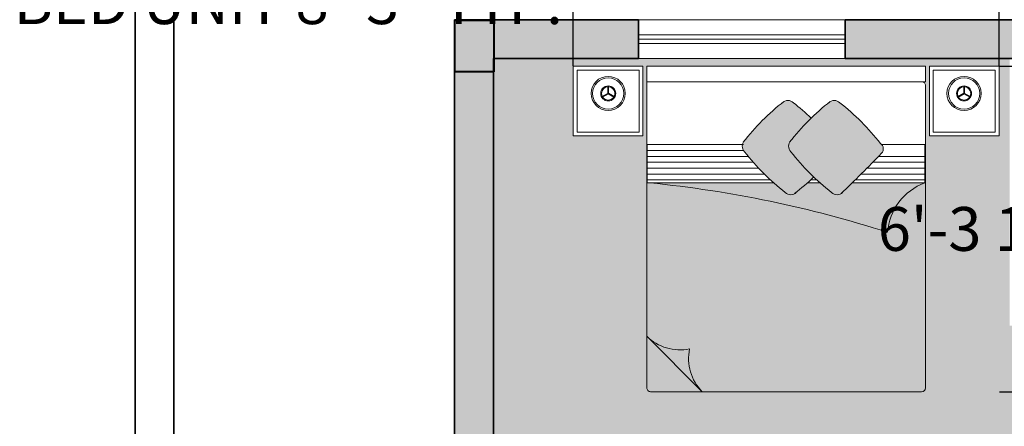
# Model space of a CAD drawing. Units: inches. Extents: x 1077 to 2505, y 1892 to 2728.
# Tile 12 of 26: x 1077 to 1306, y 2492 to 2586. Entities that reach past the tile are written whole.
import ezdxf

# ---------------------------------------------------------------- set-up
doc = ezdxf.new("R2010")
doc.units = ezdxf.units.IN
doc.linetypes.add('ACAD_ISO02W100', pattern=[15, 12, -3])
doc.layers.get('Defpoints').update_dxf_attribs({"color": 220, "linetype": 'ACAD_ISO02W100'})
for name, color, linetype, lineweight in [('00 FURNITURE', 15, 'Continuous', 15), ('A-ANNO-DIMS', 2, 'Continuous', 18), ('A-ANNO-TTLB', 7, 'Continuous', 35), ('A-COLS', 7, 'Continuous', 40), ('A-WALL-PATT', 7, 'Continuous', 9), ('WALL', 7, 'Continuous', 35), ('WINDOW', 160, 'Continuous', 13)]:
    doc.layers.add(name, color=color, linetype=linetype, lineweight=lineweight)
doc.layers.add('A-FLOR-PATT', color=254, linetype='Continuous', lineweight=9, true_color=0xd7ebd2)
doc.layers.add('A-FURN-PATT', color=177, linetype='Continuous', lineweight=9, true_color=0x293189)
doc.styles.get("Standard").update_dxf_attribs({"font": 'arial.ttf'})
doc.dimstyles.get("Standard").update_dxf_attribs({"dimtxt": 10.18, "dimasz": 0.18, "dimexe": 0.18, "dimexo": 0.0625, "dimgap": 0.09, "dimtad": 0, "dimtih": 1, "dimtoh": 1, "dimdec": 0, "dimzin": 0, "dimdsep": 46, "dimlunit": 3, "dimtxsty": 'Standard', "dimcen": 0.09, "dimadec": 0, "dimazin": 0, "dimtfac": 1, "dimtdec": 0, "dimtofl": 0, "dimtmove": 0, "dimatfit": 3, "dimfxl": 1, "dimtolj": 1, "dimtzin": 0, "dimarcsym": 0})

# ---------------------------------------------------------------- blocks, each defined once
blk = doc.blocks.new('RGWTG')
at = {"layer": '00 FURNITURE'}
for p, q in [((578.23, 3473.51), (577.36, 3475.01)), ((578.36, 3473.58), (577.49, 3475.09)), ((578.23, 3473.58), (577.36, 3472.08)), ((578.36, 3473.51), (577.49, 3472)), ((578.29, 3473.62), (580.03, 3473.62)), ((578.29, 3473.47), (580.03, 3473.47)), ((521.93, 3464.58), (509.03, 3451.68)), ((509.03, 3422.63), (509.03, 3463.68)), ((509.93, 3464.58), (566.4, 3464.58)), ((557.53, 3463.84), (557.53, 3464.49)), ((557.53, 3464.49), (566.4, 3464.49)), ((558.2, 3464.49), (558.2, 3435.82)), ((559.57, 3464.49), (559.57, 3437.25)), ((560.94, 3464.49), (560.94, 3438.58)), ((562.3, 3464.49), (562.3, 3439.83)), ((563.67, 3464.49), (563.67, 3440.99)), ((565.04, 3464.49), (565.04, 3442.08)), ((566.4, 3464.58), (580.98, 3464.58)), ((566.4, 3464.49), (566.4, 3442.08)), ((566.4, 3464.49), (566.4, 3463.84)), ((580.98, 3464.58), (580.98, 3416.72)), ((558.2, 3426.48), (558.2, 3425.04)), ((509.03, 3400.68), (509.03, 3422.63)), ((558.2, 3416.13), (558.2, 3399.95)), ((580.98, 3416.72), (580.98, 3400.68)), ((559.57, 3414.75), (559.57, 3399.95)), ((560.94, 3413.39), (560.94, 3399.95)), ((562.3, 3412.04), (562.3, 3399.95)), ((563.67, 3410.72), (563.67, 3399.95)), ((580.08, 3399.78), (509.93, 3399.78)), ((557.53, 3399.95), (557.53, 3400.6)), ((566.4, 3399.95), (557.53, 3399.95)), ((566.4, 3400.6), (566.4, 3399.95)), ((578.23, 3390.78), (577.36, 3392.29)), ((578.36, 3390.86), (577.49, 3392.36)), ((578.23, 3390.86), (577.36, 3389.36)), ((578.36, 3390.78), (577.49, 3389.28)), ((578.29, 3390.9), (580.03, 3390.9)), ((578.29, 3390.74), (580.03, 3390.74))]:
    blk.add_line(p, q, dxfattribs=at)
for points in [[(568.43, 3465.48), (584.63, 3465.48), (584.63, 3481.68), (568.43, 3481.68)], [(569.33, 3466.38), (583.73, 3466.38), (583.73, 3480.78), (569.33, 3480.78)], [(580.98, 3399.78), (584.63, 3399.78), (584.63, 3464.58), (580.98, 3464.58)], [(568.43, 3398.88), (584.63, 3398.88), (584.63, 3382.68), (568.43, 3382.68)], [(569.33, 3397.98), (583.73, 3397.98), (583.73, 3383.58), (569.33, 3383.58)]]:
    blk.add_lwpolyline(points, close=True, dxfattribs=at)
for points in [[(566.52, 3464.49), (557.53, 3464.49), (557.53, 3435.08)], [(557.53, 3427.21), (557.53, 3424.3)], [(557.53, 3416.82), (557.53, 3399.95), (566.4, 3399.95), (566.4, 3409.94)]]:
    blk.add_lwpolyline(points, dxfattribs=at)
for centre, radius in [((578.29, 3473.54), 3.97), ((578.29, 3473.54), 3.63), ((578.29, 3473.54), 1.74), ((578.29, 3473.54), 1.56), ((578.29, 3390.82), 3.97), ((578.29, 3390.82), 3.63), ((578.29, 3390.82), 1.74), ((578.29, 3390.82), 1.56)]:
    blk.add_circle(centre, radius, dxfattribs=at)
for centre, radius, start, end in [((509.93, 3463.68), 0.9, 90, 180), ((529.65, 3456.88), 10.9, 135.0361, 191.9278), ((290.56, 3490.52), 268.3, 342.2214, 354.2925), ((516.73, 3443.97), 10.9, 78.0722, 134.9639), ((566.05, 3440.57), 1.82, 45, 135), ((598.15, 3399.01), 54.32, 127.931, 142.069), ((533.58, 3399.31), 54.32, 37.931, 52.069), ((556.59, 3431.11), 1.82, 135, 225), ((598.15, 3388.23), 54.32, 127.931, 142.069), ((566.05, 3429.78), 1.82, 45, 135), ((533.58, 3388.53), 54.32, 37.931, 52.069), ((574.84, 3431.77), 1.82, 315, 45), ((597.87, 3463.6), 54.32, 217.931, 224.141), ((533.28, 3463.88), 54.32, 316.32, 322.069), ((574.84, 3420.99), 1.82, 315, 45), ((556.59, 3420.33), 1.82, 135, 225), ((533.28, 3453.1), 54.32, 307.931, 322.069), ((765.33, 3619.75), 290.45, 223.6069, 226.2326), ((545.02, 3395.29), 13.35, 20.4224, 85.5825), ((565.44, 3411.05), 1.47, 225.9674, 326.8337), ((509.93, 3400.68), 0.9, 180, 270), ((580.08, 3400.68), 0.9, 270, 0)]:
    blk.add_arc(centre, radius, start, end, dxfattribs=at)
blk = doc.blocks.new('C1')
h = blk.add_hatch(color=256)
h.dxf.hatch_style = 1
h.paths.add_polyline_path([(1668.56, 2445.41), (1677.56, 2445.41), (1677.56, 2457.41), (1668.56, 2457.41)])
for p, q in [((1668.56, 2457.41), (1677.56, 2457.41)), ((1668.56, 2445.41), (1668.56, 2457.41)), ((1677.56, 2457.41), (1677.56, 2445.41)), ((1677.56, 2445.41), (1668.56, 2445.41))]:
    blk.add_line(p, q)
blk = doc.blocks.new('WINDOW-48-EXT')
for p, q in [((0, 48), (0, 0)), ((3.5, 48), (3.5, 0)), ((4.5, 48), (4.5, 0)), ((5.5, 48), (5.5, 0)), ((9, 0), (9, 48))]:
    blk.add_line(p, q)
blk = doc.blocks.new('SHEET-FRAME-RESIDENTIAL')
for points in [[(0, 830.04), (543.52, 830.04), (543.52, 0), (0, 0)], [(9, 821.04), (534.52, 821.04), (534.52, 9), (9, 9)]]:
    blk.add_lwpolyline(points, close=True)
blk = doc.blocks.new('*D32')
at = {"layer": 'A-ANNO-DIMS', "color": 0, "lineweight": -2, "transparency": 16777216}
for p, q in [((1206.09, 2590.23), (1205.91, 2590.23)), ((1206.09, 2575.45), (1206.09, 2590.41)), ((1304.91, 2590.23), (1206.27, 2590.23)), ((1305.09, 2575.45), (1305.09, 2590.41))]:
    blk.add_line(p, q, dxfattribs=at)
at = {"layer": 'A-ANNO-DIMS', "color": 0, "transparency": 16777216}
for points in [[(1206.27, 2590.26), (1206.27, 2590.2), (1206.09, 2590.23)], [(1304.91, 2590.26), (1304.91, 2590.2), (1305.09, 2590.23)]]:
    blk.add_solid(points, dxfattribs=at)
at = {"layer": 'Defpoints', "color": 0, "transparency": 16777216}
for p in [(1206.09, 2590.23), (1206.09, 2575.38), (1305.09, 2575.38)]:
    blk.add_point(p, dxfattribs=at)
at = {"layer": 'A-ANNO-DIMS', "color": 0, "transparency": 16777216, "insert": (1139.85, 2590.23), "char_height": 10.18, "attachment_point": 5}
blk.add_mtext('\\A1;BED UNIT 8\'-3" TYP.', dxfattribs=at)
blk = doc.blocks.new('*D33')
at = {"layer": 'A-ANNO-DIMS', "color": 0, "lineweight": -2, "transparency": 16777216}
for p, q in [((1305.15, 2575.38), (1320.12, 2575.38)), ((1319.94, 2575.2), (1319.94, 2542.94)), ((1319.94, 2499.96), (1319.94, 2532.23)), ((1305.15, 2499.78), (1320.12, 2499.78))]:
    blk.add_line(p, q, dxfattribs=at)
at = {"layer": 'A-ANNO-DIMS', "color": 0, "transparency": 16777216}
for points in [[(1319.91, 2575.2), (1319.97, 2575.2), (1319.94, 2575.38)], [(1319.91, 2499.96), (1319.97, 2499.96), (1319.94, 2499.78)]]:
    blk.add_solid(points, dxfattribs=at)
at = {"layer": 'Defpoints', "color": 0, "transparency": 16777216}
for p in [(1305.09, 2575.38), (1319.94, 2575.38), (1305.09, 2499.78)]:
    blk.add_point(p, dxfattribs=at)
at = {"layer": 'A-ANNO-DIMS', "color": 0, "transparency": 16777216, "insert": (1319.94, 2537.58), "char_height": 10.18, "attachment_point": 5}
blk.add_mtext('\\A1;6\'-3 1/2" TYP.', dxfattribs=at)

msp = doc.modelspace()

# ---------------------------------------------------------------- hatches: boundary and pattern name
at = {"layer": 'A-FLOR-PATT', "transparency": 33554559}
h = msp.add_hatch(color=256, dxfattribs=at)
h.dxf.hatch_style = 1
h.paths.add_polyline_path([(1395.53, 2577.16), (1374.83, 2577.16), (1350.83, 2577.19), (1350.83, 2577.16), (1329.53, 2577.16), (1329.53, 2480.16), (1329.53, 2469.16), (1325.53, 2469.16), (1325.53, 2515.13), (1307.53, 2515.13), (1307.53, 2577.16), (1269.31, 2577.16), (1221.31, 2577.15), (1221.31, 2577.16), (1187.53, 2577.16), (1187.53, 2433.16), (1289.53, 2433.16), (1289.53, 2429.16), (1263.53, 2429.16), (1187.53, 2429.16), (1187.53, 2395.02), (1187.53, 2395.02), (1187.53, 2371.02), (1187.53, 2371.02), (1187.53, 2307.16), (1259.53, 2307.16), (1259.53, 2399.16), (1263.53, 2399.16), (1263.53, 2307.16), (1289.53, 2307.16), (1289.53, 2306.23), (1325.53, 2306.23), (1325.53, 2307.16), (1329.53, 2307.16), (1329.53, 2306.23), (1365.53, 2306.23), (1365.53, 2307.16), (1432.53, 2307.16), (1432.53, 2088.16), (1547.53, 2088.16), (1547.53, 2140.08), (1511.53, 2140.08), (1511.53, 2267.16), (1475.53, 2267.16), (1475.53, 2303.16), (1468.53, 2303.16), (1468.53, 2307.16), (1547.53, 2307.16), (1547.53, 2348.22), (1547.53, 2396.22), (1547.53, 2429.16), (1435.53, 2429.16), (1435.53, 2433.16), (1476.35, 2433.16), (1476.35, 2451.18), (1547.53, 2451.18), (1547.53, 2577.16), (1499.53, 2577.16), (1499.53, 2586.16), (1547.53, 2586.16), (1547.53, 2642.16), (1518.18, 2642.16), (1518.18, 2642.05), (1494.15, 2642.05), (1494.15, 2642.16), (1469.53, 2642.16), (1469.53, 2577.16), (1399.53, 2577.16), (1399.53, 2429.16), (1325.53, 2429.16), (1325.53, 2433.16), (1329.53, 2433.16), (1395.53, 2433.16), (1395.53, 2480.16), (1359.53, 2480.16), (1359.53, 2484.16), (1395.53, 2484.16)])
h.paths.add_polyline_path([(1357.65, 2482.07), (1355.65, 2482.07), (1355.65, 2481.07, 0.414214), (1356.65, 2480.07), (1344.65, 2480.07), (1344.65, 2477.06), (1343.27, 2477.06), (1343.27, 2480.07), (1330.65, 2480.07, -0.414214), (1329.65, 2481.07), (1329.65, 2484.07), (1331.65, 2484.07), (1331.65, 2510.07, -0.446908)], flags=16)
h.paths.add_polyline_path([(1305.09, 2559.18), (1288.89, 2559.18), (1288.89, 2575.38), (1305.09, 2575.38)], flags=16)
h.paths.add_polyline_path([(1304.19, 2560.08), (1289.79, 2560.08), (1289.79, 2574.48), (1304.19, 2574.48)], flags=0)
h.paths.add_polyline_path([(1287.99, 2500.68, -0.414214), (1287.09, 2499.78), (1265.14, 2499.78), (1224.09, 2499.78, -0.414214), (1223.19, 2500.68), (1223.19, 2557.16), (1223.19, 2571.74), (1223.19, 2575.38), (1287.99, 2575.38), (1287.99, 2571.74), (1287.09, 2571.74, -0.414214), (1287.99, 2570.84)], flags=16)
h.paths.add_polyline_path([(1292.98, 2569.05, -1), (1300.92, 2569.05, -1)], flags=0)
h.paths.add_polyline_path([(1293.32, 2569.05, -1), (1300.58, 2569.05, -1)], flags=0)
h.paths.add_polyline_path([(1322.8, 2462.21), (1322.8, 2431.71), (1323.05, 2430.71), (1323.05, 2431.71), (1321.8, 2431.71), (1321.8, 2462.19, 0.404641), (1292.3, 2431.71), (1292.05, 2430.71, -0.414214), (1291.55, 2430.21), (1291.05, 2430.21), (1291.05, 2429.71, -0.414214), (1290.55, 2429.21), (1289.55, 2429.21), (1289.55, 2434.21), (1290.55, 2434.21, -0.414214), (1291.05, 2433.71), (1291.05, 2433.21), (1291.55, 2433.21, -0.414214), (1292.05, 2432.71), (1292.3, 2431.71, -0.414214)], flags=16)
h.paths.add_polyline_path([(1287.82, 2548.28, 0.292232), (1279.17, 2536.8, 0.052719), (1223.93, 2548.28), (1223.28, 2548.28), (1223.28, 2557.16), (1223.93, 2557.16), (1245.42, 2557.16, -0.117785), (1245.77, 2557.93, -0.059418), (1254.87, 2567.02, -0.379859), (1257.28, 2566.88, -0.02509), (1261.41, 2563.32, -0.025935), (1265.65, 2567.02, -0.379859), (1268.06, 2566.88, -0.061767), (1277.52, 2557.43, -0.069393), (1277.82, 2557.16), (1287.82, 2557.16)], flags=0)
h.paths.add_polyline_path([(1263.47, 2548.28), (1260.56, 2548.28, -0.015371), (1258.01, 2546.13, -0.429576), (1255.37, 2546.06, -0.016036), (1252.69, 2548.28), (1223.28, 2548.28), (1223.28, 2554.42), (1246.78, 2554.42, 0.055344), (1255.37, 2546.06, 0.331768), (1257.52, 2545.74, 0.027343), (1262, 2549.64, 0.00919)], flags=0)
h.paths.add_polyline_path([(1295.56, 2568.34), (1296.87, 2569.09), (1296.87, 2570.6, 0.399698), (1295.39, 2569.05, 0.119004)], flags=0)
h.paths.add_polyline_path([(1295.21, 2569.05, -1), (1298.68, 2569.05, -1)], flags=0)
h.paths.add_polyline_path([(1296.95, 2568.96), (1297.03, 2569), (1297.03, 2569.09), (1296.99, 2569.11), (1296.91, 2568.98)], flags=0)
h.paths.add_polyline_path([(1402.28, 2462.19, -0.414214), (1432.78, 2431.69), (1433.03, 2432.69), (1432.78, 2431.69, 0.404641), (1403.28, 2462.17), (1403.28, 2431.69), (1402.03, 2431.69), (1402.03, 2430.69, -0.414214), (1401.53, 2430.19), (1401.03, 2430.19), (1401.03, 2429.69, -0.414214), (1400.53, 2429.19), (1399.53, 2429.19), (1399.53, 2434.19), (1400.53, 2434.19, -0.414214), (1401.03, 2433.69), (1401.03, 2433.19), (1401.53, 2433.19, -0.414214), (1402.03, 2432.69)], flags=16)
h.paths.add_polyline_path([(1470.16, 2535.21, -0.414214), (1471.06, 2536.11), (1527.54, 2536.11), (1542.12, 2536.11), (1545.76, 2536.11), (1545.76, 2471.31), (1542.12, 2471.31), (1542.12, 2472.21, -0.414214), (1541.22, 2471.31), (1471.06, 2471.31, -0.414214), (1470.16, 2472.21), (1470.16, 2494.16)], flags=16)
h.paths.add_polyline_path([(1483.07, 2536.11, 0.253465), (1480.11, 2526.15, 0.2538), (1470.15, 2523.19)], flags=16)
h.paths.add_polyline_path([(1223.19, 2512.69, 0.253465), (1233.14, 2509.74, 0.2538), (1236.1, 2499.77)], flags=16)
h.paths.add_polyline_path([(1469.77, 2578.72), (1469.77, 2581.72), (1471.77, 2581.72), (1471.77, 2607.72, -0.01951), (1473.77, 2607.68), (1473.77, 2579.72), (1473.77, 2578.72, -0.414214), (1472.77, 2577.72), (1470.77, 2577.72, -0.414214)], flags=16)
h.paths.add_polyline_path([(1382.46, 2398.13), (1395.04, 2398.13), (1395.04, 2399.74), (1382.46, 2399.74)], flags=16)
h.paths.add_polyline_path([(1379.94, 2397.18), (1379.94, 2389.82), (1380.5, 2389.82), (1380.5, 2396.05, -0.41429), (1381.06, 2396.61), (1396.47, 2396.61, -0.414213), (1397.03, 2396.05), (1397.03, 2389.82), (1397.59, 2389.82), (1397.59, 2397.18)], flags=16)
h.paths.add_polyline_path([(1263.37, 2428.14), (1263.37, 2426.14, -0.414214), (1262.37, 2425.14), (1261.37, 2425.14), (1233.41, 2425.14, 0.400854), (1259.37, 2401.04), (1259.37, 2401.14), (1261.37, 2401.14, -0.446908), (1233.37, 2427.14), (1259.37, 2427.14), (1259.37, 2429.14), (1262.37, 2429.14, -0.414214)], flags=16)
h.paths.add_polyline_path([(1404.79, 2398.13), (1417.37, 2398.13), (1417.37, 2399.74), (1404.79, 2399.74)], flags=16)
h.paths.add_polyline_path([(1402.27, 2397.18), (1404.79, 2398.13), (1417.37, 2398.13), (1419.92, 2397.18)], flags=16)
h.paths.add_polyline_path([(1432.26, 2383.16), (1432.26, 2370.59), (1433.87, 2370.59), (1433.87, 2383.16)], flags=16)
h.paths.add_polyline_path([(1431.3, 2385.69), (1423.84, 2385.69), (1423.84, 2385.13), (1430.18, 2385.13, -0.41429), (1430.74, 2384.57), (1430.74, 2369.16, -0.414237), (1430.18, 2368.6), (1423.84, 2368.6), (1423.84, 2368.03), (1431.3, 2368.03)], flags=16)
h.paths.add_polyline_path([(1417.37, 2351.16), (1417.37, 2349.54), (1418.9, 2349.54, 0.414236), (1419.92, 2350.56), (1419.92, 2352.11)], flags=16)
h.paths.add_polyline_path([(1395.04, 2351.16), (1395.04, 2349.54), (1396.58, 2349.54, 0.414235), (1397.59, 2350.56), (1397.59, 2352.11)], flags=16)
h.paths.add_polyline_path([(1366.7, 2370.05), (1365.09, 2370.05), (1365.09, 2368.52, 0.414235), (1366.11, 2367.5), (1367.66, 2367.5)], flags=16)
h.paths.add_polyline_path([(1419.36, 2359.47), (1419.36, 2353.24, -0.41419), (1418.8, 2352.68), (1403.39, 2352.68, -0.414137), (1402.83, 2353.24), (1402.83, 2359.47), (1397.03, 2359.47), (1397.03, 2353.24, -0.414189), (1396.47, 2352.68), (1381.06, 2352.68, -0.414137), (1380.5, 2353.24), (1380.5, 2359.47)], flags=16)
h.paths.add_polyline_path([(1222.29, 2559.18), (1206.09, 2559.18), (1206.09, 2575.38), (1222.29, 2575.38)], flags=16)
h.paths.add_polyline_path([(1221.39, 2560.08), (1206.99, 2560.08), (1206.99, 2574.48), (1221.39, 2574.48)], flags=0)
h.paths.add_polyline_path([(1482, 2577.72), (1482, 2580.73), (1483.38, 2580.73), (1483.38, 2577.72), (1484.77, 2577.72), (1484.77, 2574.72), (1483.38, 2574.72), (1483.38, 2577.72)], flags=16)
h.paths.add_polyline_path([(1266.37, 2415.53), (1266.37, 2414.14), (1263.37, 2414.14), (1263.37, 2415.53), (1260.36, 2415.53), (1260.36, 2416.91), (1263.37, 2416.91), (1263.37, 2415.53)], flags=16)
h.paths.add_polyline_path([(1210.26, 2569.05, -1), (1218.19, 2569.05, -1)], flags=0)
h.paths.add_polyline_path([(1210.6, 2569.05, -1), (1217.85, 2569.05, -1)], flags=0)
h.paths.add_polyline_path([(1212.84, 2568.34), (1214.15, 2569.09), (1214.15, 2570.6, 0.399698), (1212.67, 2569.05, 0.119004)], flags=0)
h.paths.add_polyline_path([(1212.49, 2569.05, -1), (1215.96, 2569.05, -1)], flags=0)
h.paths.add_polyline_path([(1214.23, 2568.96), (1214.3, 2568.91), (1214.3, 2569)], flags=0)
h.paths.add_polyline_path([(1507.18, 2480.12, 0.052719), (1518.66, 2535.36), (1518.66, 2536.01), (1527.54, 2536.01), (1527.54, 2535.36), (1527.54, 2513.88, -0.117785), (1528.31, 2513.53, -0.059418), (1537.4, 2504.43, -0.379859), (1537.26, 2502.01, -0.02509), (1533.7, 2497.89, -0.025935), (1537.4, 2493.64, -0.379859), (1537.26, 2491.23, -0.061767), (1527.8, 2481.77, -0.069393), (1527.54, 2481.47), (1527.54, 2471.47), (1518.66, 2471.47, 0.292232)], flags=0)
h.paths.add_polyline_path([(1516.43, 2503.92, -0.016036), (1518.66, 2506.6), (1518.66, 2536.01), (1524.8, 2536.01), (1524.8, 2512.51, 0.055344), (1516.43, 2503.92, 0.331768), (1516.12, 2501.77, 0.027343), (1520.01, 2497.29, 0.00919), (1518.66, 2495.82), (1518.66, 2498.73, -0.015371), (1516.5, 2501.28, -0.429576)], flags=0)
h.paths.add_polyline_path([(1499.63, 2625.5, -0.171636), (1502.82, 2631.01), (1502.82, 2633.37), (1498.68, 2633.37, -0.414214), (1497.7, 2634.36), (1497.7, 2640.66, -0.414214), (1498.68, 2641.64), (1514.82, 2641.64, -0.414214), (1515.81, 2640.66), (1515.81, 2634.36, -0.414214), (1514.82, 2633.37), (1510.69, 2633.37), (1510.69, 2631.01, -0.171636), (1513.88, 2625.5, -0.258205), (1509.31, 2614.47), (1504.19, 2614.47, -0.258205)], flags=16)
h.paths.add_polyline_path([(1501.2, 2625.5, -0.171636), (1504.39, 2631.01), (1509.12, 2631.01, -0.171636), (1512.3, 2625.5, -0.210384), (1509.35, 2616.02), (1504.16, 2616.02, -0.210384)], flags=0)
h.paths.add_polyline_path([(1529.56, 2537.01), (1529.56, 2553.21), (1545.76, 2553.21), (1545.76, 2537.01)], flags=16)
h.paths.add_polyline_path([(1530.46, 2537.91), (1530.46, 2552.31), (1544.86, 2552.31), (1544.86, 2537.91)], flags=0)
h.paths.add_polyline_path([(1535.45, 2545.07, -1), (1543.39, 2545.07, -1)], flags=0)
h.paths.add_polyline_path([(1535.8, 2545.07, -1), (1543.05, 2545.07, -1)], flags=0)
h.paths.add_polyline_path([(1529.56, 2470.41), (1545.76, 2470.41), (1545.76, 2454.21), (1529.56, 2454.21)], flags=16)
h.paths.add_polyline_path([(1541.16, 2544.99), (1540.98, 2544.99, -0.544606), (1538.71, 2543.68), (1538.62, 2543.53, 0.547962)], flags=0)
h.paths.add_polyline_path([(1530.46, 2469.51), (1544.86, 2469.51), (1544.86, 2455.11), (1530.46, 2455.11)], flags=0)
h.paths.add_polyline_path([(1539.47, 2545.14), (1539.42, 2545.22), (1539.38, 2545.14)], flags=0)
h.paths.add_polyline_path([(1543.39, 2462.34, -1), (1535.45, 2462.34, -1)], flags=0)
h.paths.add_polyline_path([(1543.05, 2462.34, -1), (1535.8, 2462.34, -1)], flags=0)
h.paths.add_polyline_path([(1541.16, 2462.27), (1540.98, 2462.27, -0.544606), (1538.71, 2460.96), (1538.62, 2460.8, 0.547962)], flags=0)
h.paths.add_polyline_path([(1539.47, 2462.42), (1539.42, 2462.5), (1539.38, 2462.42)], flags=0)
h.paths.add_polyline_path([(1435.32, 2335.25, -0.414214), (1465.82, 2304.75), (1466.07, 2305.75), (1465.82, 2304.75, 0.404641), (1436.32, 2335.23), (1436.32, 2304.75), (1435.07, 2304.75), (1435.07, 2303.75, -0.414214), (1434.57, 2303.25), (1434.07, 2303.25), (1434.07, 2302.75, -0.414214), (1433.57, 2302.25), (1432.57, 2302.25), (1432.57, 2307.25), (1433.57, 2307.25, -0.414214), (1434.07, 2306.75), (1434.07, 2306.25), (1434.57, 2306.25, -0.414214), (1435.07, 2305.75)], flags=16)
h.paths.add_polyline_path([(1532.13, 2635.71), (1535.43, 2635.71), (1535.43, 2635.89), (1532.13, 2635.89)], flags=16)
edge = h.paths.add_edge_path(flags=16)
edge.add_arc((1535.98, 2632.67), 0.183, 270, 360)
edge.add_line((1536.17, 2632.67), (1536.17, 2639.82))
edge.add_line((1536.17, 2639.82), (1538.29, 2639.82))
edge.add_line((1538.29, 2639.82), (1538.29, 2641.82))
edge.add_line((1538.29, 2641.82), (1533.25, 2641.82))
edge.add_line((1533.25, 2641.82), (1533.25, 2639.82))
edge.add_line((1533.25, 2639.82), (1534.87, 2639.82))
edge.add_line((1534.87, 2639.82), (1534.87, 2639))
edge.add_line((1534.87, 2639), (1533.7, 2639))
edge.add_line((1533.7, 2639), (1533.7, 2639.82))
edge.add_line((1533.7, 2639.82), (1533.25, 2639.82))
edge.add_line((1533.25, 2639.82), (1533.25, 2641.82))
edge.add_line((1533.25, 2641.82), (1538.29, 2641.82))
edge.add_line((1538.29, 2641.82), (1538.29, 2641.34))
edge.add_line((1538.29, 2641.34), (1540.64, 2641.58))
edge.add_line((1540.64, 2641.58), (1540.64, 2641.82))
edge.add_line((1540.64, 2641.82), (1541.5, 2641.82))
edge.add_line((1541.5, 2641.82), (1541.5, 2641.25))
edge.add_line((1541.5, 2641.25), (1541.31, 2639.79))
edge.add_ellipse((1541.09, 2638.95), major_axis=(-1.08, 0), ratio=0.790849, start_angle=180, end_angle=255.2976, ccw=False)
edge.add_line((1542.17, 2638.95), (1542.17, 2638.38))
edge.add_ellipse((1541.09, 2638.38), major_axis=(-1.08, 0), ratio=0.790849, start_angle=0, end_angle=180, ccw=False)
edge.add_line((1540, 2638.38), (1540.01, 2638.87))
edge.add_ellipse((1541.09, 2638.95), major_axis=(-1.08, 0), ratio=0.790849, start_angle=284.7024, end_angle=364.0401, ccw=False)
edge.add_line((1540.78, 2639.75), (1540.78, 2641.25))
edge.add_line((1540.78, 2641.25), (1540.64, 2641.25))
edge.add_line((1540.64, 2641.25), (1538.29, 2641.01))
edge.add_line((1538.29, 2641.01), (1538.29, 2639.82))
edge.add_line((1538.29, 2639.82), (1536.17, 2639.82))
edge.add_line((1536.17, 2639.82), (1536.17, 2632.48))
edge.add_line((1536.17, 2632.48), (1535.98, 2632.48))
h.paths.add_polyline_path([(1496.32, 2250.34, -0.292371), (1498.9, 2247.83, -0.085148), (1501.21, 2208.85, -0.01331), (1500.27, 2098.5, -0.379287), (1497.22, 2095.28, -0.0502), (1441.54, 2095.28, -0.379287), (1438.5, 2098.5, -0.01331), (1437.56, 2208.85, -0.086132), (1439.96, 2248.26, -0.295116), (1442.59, 2250.78, -0.114238)], flags=16)
h.paths.add_polyline_path([(1495.16, 2205.84, -0.355389), (1496.7, 2202.1), (1492.94, 2189.65, -0.398275), (1489.12, 2187.47, 0.113332), (1449.64, 2187.47, -0.398275), (1445.82, 2189.65), (1442.06, 2202.1, -0.355394), (1443.6, 2205.84, -0.265725)], flags=0)
h.paths.add_polyline_path([(1440.37, 2195.72), (1445.94, 2181.67), (1445.94, 2160.63), (1440.84, 2157.26)], flags=0)
h.paths.add_polyline_path([(1498.46, 2195.72), (1497.99, 2157.26), (1492.88, 2160.63), (1492.88, 2181.67)], flags=0)
h.paths.add_polyline_path([(1445.94, 2158.37), (1445.94, 2137.12), (1441.12, 2122.56), (1440.87, 2155.03)], flags=0)
h.paths.add_polyline_path([(1492.88, 2158.37), (1497.96, 2155.03), (1497.71, 2122.56), (1492.88, 2137.12)], flags=0)
h.paths.add_polyline_path([(1489.88, 2130.4), (1494.39, 2107.67, -0.090102), (1444.44, 2107.65), (1448.95, 2130.39, 0.036636)], flags=0)
h.paths.add_polyline_path([(1447.54, 2159.34), (1497.44, 2159.34), (1497.44, 2177.89), (1447.54, 2177.89)], flags=8)
h.paths.add_polyline_path([(1196.44, 2354.84), (1246.65, 2354.84), (1246.65, 2388.43), (1196.44, 2388.43)], flags=24)
h.paths.add_polyline_path([(1296.09, 2360.25), (1353.81, 2360.25), (1353.81, 2393.84), (1296.09, 2393.84)], flags=24)
h.paths.add_polyline_path([(1400.72, 2471.85), (1470.63, 2471.85), (1470.63, 2505.44), (1400.72, 2505.44)], flags=24)
h.paths.add_polyline_path([(1324.78, 2448.48), (1394.95, 2448.48), (1394.95, 2467.02), (1324.78, 2467.02)], flags=24)
h.paths.add_polyline_path([(1335.08, 2531.43), (1389.67, 2531.43), (1389.67, 2565.02), (1335.08, 2565.02)], flags=24)
h.paths.add_polyline_path([(1225.76, 2460), (1295.67, 2460), (1295.67, 2493.58), (1225.76, 2493.58)], flags=24)
h = msp.add_hatch(color=256, dxfattribs=at)
h.dxf.hatch_style = 1
h.paths.add_polyline_path([(1547.53, 2348.22), (1547.53, 2396.22), (1547.53, 2425.11), (1547.53, 2425.11), (1547.53, 2429.16), (1435.53, 2429.16), (1434.03, 2429.21), (1434.03, 2430.19), (1433.03, 2430.19), (1432.78, 2431.69, 0.404641), (1403.28, 2462.17), (1403.28, 2431.69), (1402.03, 2431.69), (1402.03, 2430.19), (1401.03, 2430.19), (1401.03, 2429.19), (1399.53, 2429.19), (1399.53, 2429.19), (1399.53, 2429.16), (1334.67, 2429.16), (1334.67, 2423.95), (1325.67, 2423.95), (1325.67, 2429.16), (1325.53, 2429.16), (1324.05, 2429.24), (1324.05, 2430.21), (1323.05, 2430.21), (1323.05, 2431.71), (1321.8, 2431.71), (1321.8, 2462.19, 0.416544), (1292.05, 2430.73, -0.423614), (1291.55, 2430.21), (1291.05, 2430.21), (1291.05, 2429.21), (1289.55, 2429.21), (1289.53, 2429.21), (1289.53, 2429.16), (1263.37, 2429.16), (1263.37, 2415.53), (1266.37, 2415.53), (1266.37, 2414.14), (1263.37, 2414.14), (1263.37, 2399.16), (1263.53, 2399.16), (1263.53, 2307.16), (1289.53, 2307.16), (1289.53, 2306.23), (1323.26, 2306.23), (1323.26, 2307.21), (1332.26, 2307.21), (1365.53, 2306.23), (1365.53, 2307.16), (1432.53, 2307.16), (1432.57, 2307.16), (1432.57, 2307.25), (1434.07, 2307.25), (1434.07, 2306.25), (1435.32, 2306.25), (1435.32, 2335.25, -0.407346), (1466.07, 2305.73, -0.423614), (1466.57, 2306.25), (1467.07, 2306.25), (1467.07, 2307.25), (1468.57, 2307.25), (1547.53, 2307.16), (1547.53, 2307.2)])
h.paths.add_polyline_path([(1430.74, 2369.16), (1430.74, 2384.57, 0.41429), (1430.18, 2385.13), (1423.84, 2385.13), (1423.84, 2368.6), (1430.18, 2368.6, 0.414237)], flags=16)
h.paths.add_polyline_path([(1432.26, 2383.16), (1432.26, 2370.59), (1433.87, 2370.59), (1433.87, 2383.16)], flags=16)
h.paths.add_polyline_path([(1431.3, 2368.03), (1431.3, 2385.69), (1432.26, 2383.16), (1432.26, 2370.59)], flags=16)
h.paths.add_polyline_path([(1417.37, 2351.16), (1417.37, 2349.54), (1418.9, 2349.54, 0.414236), (1419.92, 2350.56), (1419.92, 2352.11)], flags=16)
h.paths.add_polyline_path([(1403.39, 2352.68), (1418.78, 2352.68, 0.42427), (1419.36, 2353.24), (1419.36, 2359.47), (1402.83, 2359.47), (1402.83, 2353.24, 0.414137)], flags=16)
h.paths.add_polyline_path([(1366.7, 2370.05), (1365.09, 2370.05), (1365.09, 2368.52, 0.414235), (1366.11, 2367.5), (1367.66, 2367.5)], flags=16)
h.paths.add_polyline_path([(1382.46, 2398.13), (1395.04, 2398.13), (1395.04, 2399.74), (1382.46, 2399.74)], flags=16)
h.paths.add_polyline_path([(1396.47, 2396.61), (1381.06, 2396.61, 0.41429), (1380.5, 2396.05), (1380.5, 2389.82), (1397.03, 2389.82), (1397.03, 2396.05, 0.414213)], flags=16)
h.paths.add_polyline_path([(1402.27, 2397.18), (1402.83, 2396.05, -0.414213), (1403.39, 2396.61)], flags=16)
h.paths.add_polyline_path([(1418.8, 2396.61), (1419.36, 2396.61), (1419.36, 2396.05, 0.414237)], flags=16)
h.paths.add_polyline_path([(1404.79, 2398.13), (1417.37, 2398.13), (1417.37, 2399.74), (1404.79, 2399.74)], flags=16)
h.paths.add_polyline_path([(1381.06, 2352.68, -0.414213), (1380.5, 2353.24), (1380.27, 2352.11)], flags=16)
h.paths.add_polyline_path([(1396.58, 2349.54), (1396.58, 2349.54), (1395.04, 2349.54), (1395.04, 2349.54), (1382.46, 2349.54), (1382.46, 2351.16), (1395.04, 2351.16), (1397.59, 2352.11), (1397.59, 2350.56, -0.414235)], flags=16)
h.paths.add_polyline_path([(1379.94, 2397.18), (1382.46, 2398.13), (1395.04, 2398.13), (1397.59, 2397.18)], flags=16)
h.paths.add_polyline_path([(1368.78, 2384.59, 0.414213), (1368.22, 2384.03), (1367.66, 2367.5), (1367.66, 2385.15)], flags=16)
h.paths.add_polyline_path([(1547.53, 2574.38), (1547.51, 2574.38), (1547.51, 2577.16), (1499.53, 2577.16), (1484.77, 2577.44), (1484.77, 2574.72), (1483.38, 2574.72), (1483.38, 2577.72), (1482, 2577.72), (1469.53, 2577.72), (1469.53, 2577.16), (1401.95, 2577.16), (1401.95, 2574.12), (1399.53, 2574.12), (1399.53, 2434.19), (1401.03, 2434.19), (1401.03, 2433.19), (1402.28, 2433.19), (1402.28, 2462.19, -0.407346), (1433.03, 2432.67, -0.423614), (1433.53, 2433.19), (1434.03, 2433.19), (1434.03, 2434.19), (1435.53, 2434.19), (1476.35, 2433.81), (1476.35, 2451.18), (1547.53, 2451.18)])
h.paths.add_polyline_path([(1470.16, 2535.21, -0.414214), (1471.06, 2536.11), (1527.54, 2536.11), (1542.12, 2536.11), (1545.76, 2536.11), (1545.76, 2471.31), (1542.12, 2471.31), (1542.12, 2472.21, -0.414214), (1541.22, 2471.31), (1471.06, 2471.31, -0.414214), (1470.16, 2472.21), (1470.16, 2494.16)], flags=16)
h.paths.add_polyline_path([(1483.07, 2536.11, 0.253465), (1480.11, 2526.15, 0.2538), (1470.15, 2523.19)], flags=16)
h.paths.add_polyline_path([(1525.55, 2481.52, -0.000893), (1524.8, 2482.24), (1524.8, 2471.47), (1527.54, 2471.47), (1527.54, 2472.12), (1527.54, 2481.47, -0.388819)], flags=0)
h.paths.add_polyline_path([(1518.66, 2536.01), (1527.54, 2536.01), (1527.54, 2535.36), (1527.54, 2513.88, -0.117785), (1528.31, 2513.53, -0.059418), (1537.4, 2504.43, -0.379859), (1537.26, 2502.01, -0.02509), (1533.7, 2497.89, 0.033431), (1528.3, 2502.74, 0.308459), (1526.25, 2502.88, 0.047827), (1518.66, 2495.82), (1518.66, 2498.73, -0.015371), (1516.5, 2501.28, -0.429576), (1516.43, 2503.92, -0.016036), (1518.66, 2506.6)], flags=0)
h.paths.add_polyline_path([(1529.56, 2537.01), (1529.56, 2553.21), (1545.76, 2553.21), (1545.76, 2537.01)], flags=16)
h.paths.add_polyline_path([(1530.46, 2537.91), (1530.46, 2552.31), (1544.86, 2552.31), (1544.86, 2537.91)], flags=0)
h.paths.add_polyline_path([(1535.8, 2545.07, -1), (1543.05, 2545.07, -1)], flags=0)
h.paths.add_polyline_path([(1541.16, 2544.99), (1540.98, 2544.99, -0.544606), (1538.71, 2543.68), (1538.62, 2543.53, 0.547962)], flags=0)
h.paths.add_polyline_path([(1539.47, 2545.14), (1539.42, 2545.22), (1539.38, 2545.14)], flags=0)
h.paths.add_polyline_path([(1529.56, 2470.41), (1545.76, 2470.41), (1545.76, 2454.21), (1529.56, 2454.21)], flags=16)
h.paths.add_polyline_path([(1530.46, 2469.51), (1544.86, 2469.51), (1544.86, 2455.11), (1530.46, 2455.11)], flags=0)
h.paths.add_polyline_path([(1535.8, 2462.34, -1), (1543.05, 2462.34, -1)], flags=0)
h.paths.add_polyline_path([(1541.16, 2462.27), (1540.98, 2462.27, -0.544606), (1538.71, 2460.96), (1538.62, 2460.8, 0.547962)], flags=0)
h.paths.add_polyline_path([(1539.47, 2462.42), (1539.42, 2462.5), (1539.38, 2462.42)], flags=0)
h.paths.add_polyline_path([(1395.53, 2574.12), (1392.95, 2574.12), (1392.95, 2577.16), (1374.83, 2577.16), (1350.83, 2577.19), (1350.83, 2577.16), (1332.07, 2577.16), (1332.07, 2574), (1329.53, 2574), (1329.53, 2484.07), (1331.65, 2484.07), (1331.65, 2510.07, -0.423677), (1357.76, 2484.07), (1359.53, 2484.07), (1359.53, 2484.16), (1395.53, 2484.16)], flags=17)
h.paths.add_polyline_path([(1395.53, 2480.16), (1359.06, 2480.16, 0.437533), (1359.53, 2481.55), (1359.53, 2484.16), (1395.53, 2484.16), (1395.53, 2574.12), (1392.95, 2574.12), (1392.95, 2577.16), (1374.83, 2577.16), (1350.83, 2577.19), (1350.83, 2577.16), (1332.07, 2577.16), (1332.07, 2574), (1329.53, 2574), (1329.53, 2484.07), (1329.65, 2484.07), (1329.65, 2481.07), (1329.53, 2480.16), (1329.53, 2469.16), (1325.53, 2469.16), (1325.53, 2515.13), (1307.53, 2515.13), (1307.53, 2577.16), (1269.31, 2577.16), (1221.31, 2577.15), (1221.31, 2577.16), (1187.61, 2577.16), (1187.61, 2574.03), (1187.53, 2433.16), (1289.55, 2433.16), (1289.55, 2434.21), (1291.05, 2434.21), (1291.05, 2433.21), (1292.05, 2433.21), (1292.3, 2431.71, -0.414214), (1322.8, 2462.21), (1323.05, 2432.71, -0.414214), (1323.55, 2433.21), (1324.05, 2433.21), (1324.05, 2434.21), (1325.67, 2434.21), (1325.67, 2435.95), (1334.67, 2435.95), (1334.67, 2433.16), (1395.53, 2433.16)])
h.paths.add_polyline_path([(1344.65, 2480.07), (1344.65, 2477.06), (1343.27, 2477.06), (1343.27, 2480.07), (1332.65, 2480.07, 0.414214), (1333.65, 2481.07), (1333.65, 2482.07), (1331.65, 2482.07), (1331.65, 2484.07), (1331.65, 2510.07, -0.446908), (1357.65, 2482.07), (1355.65, 2482.07), (1355.65, 2481.07, 0.414214), (1356.65, 2480.07)], flags=16)
h.paths.add_polyline_path([(1287.99, 2500.68, -0.414214), (1287.09, 2499.78), (1265.14, 2499.78), (1224.09, 2499.78, -0.414214), (1223.19, 2500.68), (1223.19, 2557.16), (1223.19, 2571.74), (1223.19, 2575.38), (1287.99, 2575.38), (1287.99, 2571.74), (1287.09, 2571.74, -0.414214), (1287.99, 2570.84)], flags=16)
h.paths.add_polyline_path([(1277.77, 2555.17, -0.000893), (1277.05, 2554.42), (1287.82, 2554.42), (1287.82, 2557.16), (1287.17, 2557.16), (1277.82, 2557.16, -0.388819)], flags=0)
h.paths.add_polyline_path([(1223.28, 2548.28), (1223.28, 2557.16), (1223.93, 2557.16), (1245.42, 2557.16, -0.117785), (1245.77, 2557.93, -0.059418), (1254.87, 2567.02, -0.379859), (1257.28, 2566.88, -0.02509), (1261.41, 2563.32, 0.033431), (1256.55, 2557.93, 0.308459), (1256.41, 2555.88, 0.047827), (1263.47, 2548.28), (1260.56, 2548.28, -0.015371), (1258.01, 2546.13, -0.429576), (1255.37, 2546.06, -0.016036), (1252.69, 2548.28)], flags=0)
h.paths.add_polyline_path([(1305.09, 2559.18), (1288.89, 2559.18), (1288.89, 2575.38), (1305.09, 2575.38)], flags=16)
h.paths.add_polyline_path([(1304.19, 2560.08), (1289.79, 2560.08), (1289.79, 2574.48), (1304.19, 2574.48)], flags=0)
h.paths.add_polyline_path([(1300.58, 2569.05, -1), (1293.32, 2569.05, -1)], flags=0)
h.paths.add_polyline_path([(1223.19, 2512.69, 0.253465), (1233.14, 2509.74, 0.2538), (1236.1, 2499.77)], flags=16)
h.paths.add_polyline_path([(1295.56, 2568.34), (1296.87, 2569.09), (1296.87, 2570.6, 0.399698), (1295.39, 2569.05, 0.119004)], flags=0)
h.paths.add_polyline_path([(1295.21, 2569.05, -1), (1298.68, 2569.05, -1)], flags=0)
h.paths.add_polyline_path([(1296.95, 2568.96), (1297.03, 2569), (1297.03, 2569.09), (1296.99, 2569.11), (1296.91, 2568.98)], flags=0)
h.paths.add_polyline_path([(1222.29, 2559.18), (1206.09, 2559.18), (1206.09, 2575.38), (1222.29, 2575.38)], flags=16)
h.paths.add_polyline_path([(1221.39, 2560.08), (1206.99, 2560.08), (1206.99, 2574.48), (1221.39, 2574.48)], flags=0)
h.paths.add_polyline_path([(1217.85, 2569.05, -1), (1210.6, 2569.05, -1)], flags=0)
h.paths.add_polyline_path([(1212.84, 2568.34), (1214.15, 2569.09), (1214.15, 2570.6, 0.399698), (1212.67, 2569.05, 0.119004)], flags=0)
h.paths.add_polyline_path([(1212.49, 2569.05, -1), (1215.96, 2569.05, -1)], flags=0)
h.paths.add_polyline_path([(1214.23, 2568.96), (1214.3, 2569), (1214.3, 2569.09), (1214.26, 2569.11), (1214.19, 2568.98)], flags=0)
h.paths.add_polyline_path([(1259.53, 2399.14), (1259.37, 2399.14), (1259.37, 2401.04, -0.423677), (1233.37, 2427.14), (1259.37, 2427.14), (1259.37, 2429.16), (1187.53, 2429.16), (1187.53, 2395.02), (1187.53, 2395.02), (1187.53, 2371.02), (1187.53, 2371.02), (1187.53, 2311.49), (1187.55, 2311.49), (1187.55, 2307.16), (1259.53, 2307.16)])
h.paths.add_polyline_path([(1323.26, 2295.21), (1323.26, 2304.23), (1289.53, 2304.23), (1289.53, 2303.16), (1187.55, 2303.16), (1187.55, 2299.49), (1178.53, 2299.49), (1178.53, 2267.66), (1178.53, 2219.66), (1182.03, 2219.66), (1182.03, 2267.67), (1184.03, 2267.67), (1184.03, 2219.66), (1187.53, 2219.66), (1187.53, 2153.16), (1228.13, 2153.16), (1276.13, 2153.16), (1276.13, 2153.16), (1324.54, 2153.16), (1324.54, 2154.67), (1325.54, 2154.67), (1325.54, 2155.92), (1296.54, 2155.92, -0.407346), (1326.06, 2186.67, -0.423614), (1325.54, 2187.17), (1325.54, 2187.67), (1324.54, 2187.67), (1324.54, 2189.17), (1325.43, 2295.21)])
h.paths.add_polyline_path([(1432.53, 2307.16), (1365.53, 2307.16), (1365.53, 2306.23), (1365.53, 2303.16), (1428.53, 2303.16), (1428.53, 2221.2), (1428.57, 2221.2), (1428.57, 2197.2), (1428.53, 2197.16), (1428.53, 2303.01), (1404.46, 2303.01), (1404.46, 2221.2), (1329.53, 2221.2), (1329.53, 2307.16), (1325.53, 2307.16), (1325.53, 2295.21), (1325.43, 2295.21), (1324.54, 2189.17), (1324.54, 2187.67), (1326.04, 2187.67, 1.016365), (1326.06, 2186.67, 0.407348), (1296.54, 2155.92), (1325.54, 2155.92), (1325.54, 2154.67), (1324.54, 2154.67), (1324.54, 2153.16), (1329.53, 2153.16), (1329.53, 2144.16), (1432.53, 2144.16)])
h.paths.add_polyline_path([(1361.95, 2194.26), (1361.95, 2193.16), (1329.53, 2193.16), (1329.53, 2189.16), (1329.54, 2188.17), (1329.54, 2189.16), (1329.53, 2189.16), (1329.53, 2193.16), (1361.95, 2193.16), (1361.95, 2196.26), (1409.95, 2196.26), (1409.95, 2194.26)], flags=16)
h.paths.add_polyline_path([(1377.02, 2200.5), (1345.91, 2200.5), (1345.91, 2218.4), (1347.87, 2218.4), (1347.87, 2219.18), (1374.75, 2219.18), (1374.75, 2218.4), (1377.02, 2218.4)], flags=16)
h.paths.add_polyline_path([(1367.07, 2210.7, -1), (1373.34, 2210.7, -1)], flags=0)
h.paths.add_polyline_path([(1349.92, 2210.7, -1), (1356.98, 2210.7, -1)], flags=0)
h.paths.add_polyline_path([(1405.95, 2256.57), (1405.95, 2277.6), (1427.86, 2277.6), (1427.86, 2256.57)], flags=16)
h.paths.add_polyline_path([(1412.92, 2258.68, -0.414201), (1410.93, 2260.67), (1410.93, 2273.62, -0.414239), (1412.92, 2275.61), (1423.88, 2275.61, -0.414227), (1425.87, 2273.62), (1425.87, 2260.67, -0.414214), (1423.88, 2258.68)], flags=0)
h.paths.add_polyline_path([(1407.61, 2263.66, -1), (1409.18, 2263.66, -1)], flags=0)
h.paths.add_polyline_path([(1407.61, 2267.14, -1), (1409.18, 2267.14, -1)], flags=0)
h.paths.add_polyline_path([(1416.91, 2267.15, -1), (1419.89, 2267.15, -1)], flags=0)
h.paths.add_polyline_path([(1407.61, 2270.63, -1), (1409.18, 2270.63, -1)], flags=0)
h.paths.add_polyline_path([(1475.53, 2303.16), (1468.57, 2303.16), (1468.57, 2302.25), (1467.07, 2302.25), (1467.07, 2303.25), (1466.07, 2303.25), (1465.82, 2304.75, 0.404641), (1436.32, 2335.23), (1436.32, 2304.75), (1435.07, 2304.75), (1435.07, 2303.25), (1434.07, 2303.25), (1434.07, 2302.25), (1432.53, 2302.25), (1432.53, 2144.16), (1432.53, 2088.16), (1547.52, 2088.16), (1547.52, 2100.19), (1547.52, 2140.08), (1511.53, 2140.08), (1511.53, 2267.16), (1475.53, 2267.16)])
h.paths.add_polyline_path([(1438.35, 2102.86, 0.033498), (1438.37, 2102.21, -0.000079)], flags=16)
h.paths.add_polyline_path([(1496.32, 2250.34, -0.292371), (1498.9, 2247.83, -0.085148), (1501.21, 2208.85, -0.012784), (1500.42, 2102.86, -0.033498), (1500.39, 2102.21, 0.012863), (1501.21, 2208.85, 0.077283), (1499.67, 2244.3, 0.265882), (1497.48, 2246.8, 0.14401), (1441.46, 2247.36, 0.270646), (1439.21, 2244.85, -0.007564), (1439.96, 2248.26, -0.295116), (1442.59, 2250.78, -0.114238)], flags=16)
h.paths.add_polyline_path([(1495.16, 2205.84, -0.355389), (1496.7, 2202.1), (1492.94, 2189.65, -0.398275), (1489.12, 2187.47, 0.113332), (1449.64, 2187.47, -0.398275), (1445.82, 2189.65), (1442.06, 2202.1, -0.355394), (1443.6, 2205.84, -0.265725)], flags=16)
h.paths.add_polyline_path([(1440.37, 2195.72), (1445.94, 2181.67), (1445.94, 2160.63), (1440.84, 2157.26)], flags=16)
h.paths.add_polyline_path([(1498.46, 2195.72), (1497.99, 2157.26), (1492.88, 2160.63), (1492.88, 2181.67)], flags=16)
h.paths.add_polyline_path([(1445.94, 2158.37), (1445.94, 2137.12), (1441.12, 2122.56), (1440.87, 2155.03)], flags=16)
h.paths.add_polyline_path([(1492.88, 2158.37), (1497.96, 2155.03), (1497.71, 2122.56), (1492.88, 2137.12)], flags=16)
h.paths.add_polyline_path([(1489.88, 2130.4), (1494.39, 2107.67, -0.090102), (1444.44, 2107.65), (1448.95, 2130.39, 0.036636)], flags=16)
h.paths.add_polyline_path([(1296.09, 2360.25), (1353.81, 2360.25), (1353.81, 2393.84), (1296.09, 2393.84)], flags=24)
h.paths.add_polyline_path([(1400.72, 2471.85), (1470.63, 2471.85), (1470.63, 2505.44), (1400.72, 2505.44)], flags=24)
h.paths.add_polyline_path([(1335.08, 2531.43), (1389.67, 2531.43), (1389.67, 2565.02), (1335.08, 2565.02)], flags=24)
h.paths.add_polyline_path([(1324.78, 2448.48), (1394.95, 2448.48), (1394.95, 2467.02), (1324.78, 2467.02)], flags=24)
h.paths.add_polyline_path([(1225.76, 2460), (1295.67, 2460), (1295.67, 2493.58), (1225.76, 2493.58)], flags=24)
h.paths.add_polyline_path([(1196.44, 2354.84), (1246.65, 2354.84), (1246.65, 2388.43), (1196.44, 2388.43)], flags=24)
h.paths.add_polyline_path([(1447.54, 2159.34), (1497.44, 2159.34), (1497.44, 2177.89), (1447.54, 2177.89)], flags=24)
at = {"layer": 'A-FURN-PATT', "transparency": 33554610}
h = msp.add_hatch(color=256, dxfattribs=at)
h.dxf.hatch_style = 1
h.paths.add_polyline_path([(1287.99, 2548.28), (1287.82, 2548.28, 0.292232), (1279.17, 2536.8, 0.052719), (1223.93, 2548.28), (1223.19, 2548.28), (1223.19, 2512.69, 0.253465), (1233.14, 2509.74, 0.253465), (1236.09, 2499.78), (1265.14, 2499.78), (1287.09, 2499.78, 0.414214), (1287.99, 2500.68)])
h.paths.add_polyline_path([(1223.19, 2512.69), (1223.19, 2500.68, 0.414214), (1224.09, 2499.78), (1236.09, 2499.78)], flags=17)
h.paths.add_polyline_path([(1277.52, 2557.43, 0.061767), (1268.06, 2566.88, 0.380465), (1265.65, 2567.03, 0.059418), (1256.55, 2557.93, 0.379859), (1256.7, 2555.51, 0.061767), (1266.15, 2546.06, 0.334836), (1268.32, 2545.75, 0.011497), (1277.78, 2555.18, 0.468078)])
h.paths.add_polyline_path([(1256.55, 2557.93, -0.033431), (1261.41, 2563.32, 0.025099), (1257.28, 2566.88, 0.380465), (1254.86, 2567.03, 0.059418), (1245.77, 2557.93, 0.379859), (1245.91, 2555.51, 0.061767), (1255.37, 2546.06, 0.331768), (1257.52, 2545.74, 0.027343), (1262, 2549.64, -0.036481), (1256.7, 2555.51, -0.379859)])
h.paths.add_polyline_path([(1287.82, 2548.28), (1270.95, 2548.28, -0.003141), (1268.32, 2545.75, -0.334836), (1266.15, 2546.06, -0.016036), (1263.47, 2548.28), (1260.56, 2548.28, -0.015371), (1258.01, 2546.13, -0.429576), (1255.37, 2546.06, -0.016036), (1252.69, 2548.28), (1223.93, 2548.28, -0.052719), (1279.17, 2536.8, -0.292232)], flags=17)
at = {"layer": 'A-WALL-PATT', "transparency": 33554585}
h = msp.add_hatch(color=256, dxfattribs=at)
h.dxf.hatch_style = 1
h.paths.add_polyline_path([(1187.53, 2424), (1178.53, 2424), (1178.53, 2395.02), (1187.53, 2395.02)])
h.paths.add_polyline_path([(1187.53, 2371.02), (1178.53, 2371.02), (1178.53, 2311.49), (1187.53, 2311.49)])
h.paths.add_polyline_path([(1228.13, 2153.16), (1187.53, 2153.16), (1187.53, 2219.66), (1178.53, 2219.66), (1178.53, 2100.18), (1187.53, 2100.18), (1187.53, 2144.16), (1228.13, 2144.16)])
h.paths.add_polyline_path([(1432.53, 2097.16), (1187.53, 2097.16), (1187.53, 2100.18), (1178.53, 2100.18), (1178.53, 2088.16), (1432.53, 2088.16)])
h.paths.add_polyline_path([(1556.53, 2348.22), (1547.53, 2348.22), (1547.53, 2348.22), (1547.53, 2307.16), (1468.53, 2307.16), (1468.53, 2303.16), (1547.53, 2303.16), (1547.53, 2088.16), (1556.53, 2088.16)])
h.paths.add_polyline_path([(1556.53, 2425.11), (1547.53, 2425.11), (1547.53, 2396.22), (1556.53, 2396.22)])
h.paths.add_polyline_path([(1547.53, 2433.16), (1435.53, 2433.16), (1435.53, 2429.16), (1547.53, 2429.16)])
h.paths.add_polyline_path([(1556.53, 2574.38), (1547.53, 2574.38), (1547.53, 2451.18), (1547.55, 2451.18), (1547.55, 2437.11), (1556.53, 2437.11)])
h.paths.add_polyline_path([(1556.53, 2639.11), (1547.53, 2639.11), (1547.53, 2586.38), (1556.53, 2586.38)])
h.paths.add_polyline_path([(1556.53, 2639.11), (1547.53, 2639.11), (1547.53, 2642.16), (1518.18, 2642.16), (1518.18, 2642.05), (1494.18, 2642.05), (1494.18, 2651.05), (1518.15, 2651.05), (1518.15, 2651.16), (1556.53, 2651.16)])
h.paths.add_polyline_path([(1494.15, 2651.16), (1469.6, 2651.16), (1469.6, 2642.16), (1494.15, 2642.16)])
h.paths.add_polyline_path([(1221.31, 2577.16), (1187.61, 2577.16), (1187.61, 2574.03), (1178.61, 2574.03), (1178.61, 2586.16), (1221.31, 2586.16)])
h.paths.add_polyline_path([(1323.07, 2586.16), (1269.31, 2586.16), (1269.31, 2577.16), (1323.07, 2577.16)])
h.paths.add_polyline_path([(1374.84, 2586.19), (1374.84, 2577.19), (1350.84, 2577.19), (1350.83, 2577.19), (1350.83, 2577.16), (1332.07, 2577.16), (1332.07, 2574), (1323.07, 2574), (1323.07, 2586.16), (1350.83, 2586.16), (1350.84, 2586.16), (1350.84, 2586.19)])
h.paths.add_polyline_path([(1392.95, 2586.16), (1374.84, 2586.16), (1374.84, 2577.16), (1392.95, 2577.16)], flags=17)
h.paths.add_polyline_path([(1469.53, 2642.16), (1469.6, 2651.16), (1460.53, 2651.16), (1460.53, 2586.16), (1392.95, 2586.16), (1392.95, 2577.16), (1395.53, 2577.16), (1395.53, 2484.16), (1359.53, 2484.16), (1359.53, 2480.16), (1395.53, 2480.16), (1395.53, 2433.16), (1329.53, 2433.16), (1325.53, 2433.16), (1325.53, 2429.16), (1399.53, 2429.16), (1399.53, 2577.16), (1469.53, 2577.16)])
h.paths.add_polyline_path([(1187.53, 2574.03), (1178.53, 2574.03), (1178.53, 2436), (1187.53, 2436)])

# ---------------------------------------------------------------- linework, layer by layer
at = {"layer": 'WALL'}
for p, q in [((1178.53, 2586.16), (1221.31, 2586.16)), ((1178.53, 2395.02), (1178.53, 2586.16)), ((1221.31, 2577.16), (1221.31, 2586.16)), ((1269.31, 2577.16), (1269.31, 2586.16)), ((1269.31, 2586.16), (1350.83, 2586.16)), ((1187.53, 2577.16), (1221.31, 2577.16)), ((1187.53, 2433.16), (1187.53, 2577.16)), ((1269.31, 2577.16), (1325.53, 2577.16))]:
    msp.add_line(p, q, dxfattribs=at)

# ---------------------------------------------------------------- block references
at = {"layer": '00 FURNITURE', "rotation": 89.99999999999999}
msp.add_blockref('RGWTG', (4687.77, 1990.75), dxfattribs=at)
at = {"layer": 'A-ANNO-TTLB'}
msp.add_blockref('SHEET-FRAME-RESIDENTIAL', (1104.25, 1892.27), dxfattribs=at)
at = {"layer": 'A-COLS'}
msp.add_blockref('C1', (-489.95, 128.62), dxfattribs=at)
at = {"layer": 'WINDOW', "rotation": 89.99999999999928}
msp.add_blockref('WINDOW-48-EXT', (1269.32, 2577.15), dxfattribs=at)

# ---------------------------------------------------------------- dimensions: what is measured, and where the dimension line sits
at = {"layer": 'A-ANNO-DIMS'}
for base, p1, p2, angle, text, picture, middle in [((1206.09, 2590.23), (1305.09, 2575.38), (1206.09, 2575.38), 180, 'BED UNIT <> TYP.', '*D32', (1139.85, 2590.23)), ((1319.94, 2575.38), (1305.09, 2499.78), (1305.09, 2575.38), 90, '<> TYP.', '*D33', (1319.94, 2537.58))]:
    dim = msp.add_linear_dim(base=base, p1=p1, p2=p2, angle=angle, text=text, dimstyle='Standard', override={"dimdec": 1, "dimlfac": 1, "dimrnd": 0, "dimzin": 1, "dimdsep": 46, "dimlunit": 4, "dimfrac": 2}, dxfattribs=at)
    dim.commit()
    dim.dimension.update_dxf_attribs({"geometry": picture, "text_midpoint": middle})

doc.saveas('drawing.dxf')
